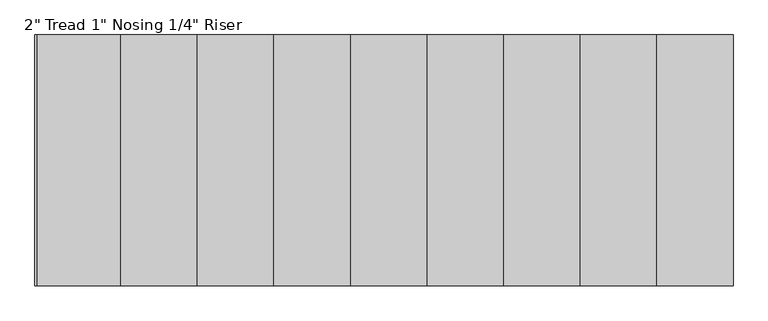
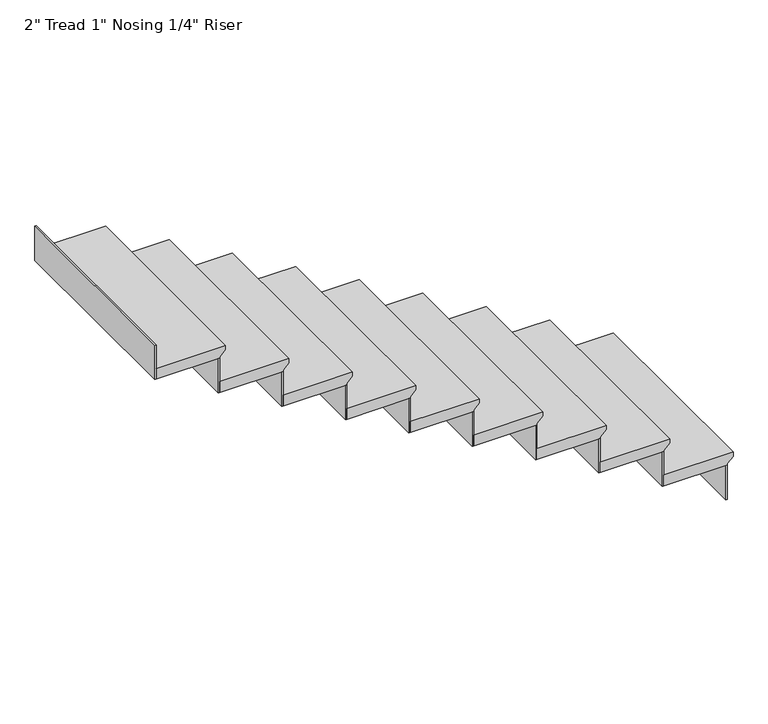
"""IFC4 building model written with IfcOpenShell, lengths in millimetres: stair flight geometry."""

from ifc_helpers import new_model, si_unit, frame, origin, place, context, project, spatial, polyline, outline, extrude, source, transform, mapped, element, save


def stair_flight_035a5224(model_context):
    return source(origin(), model_context, "Body", "SweptSolid", [
        extrude(outline(polyline([(1760.22, 923.4845537), (1760.22, 618.6845537), (1709.42, 618.6845537), (1709.42, 898.0845537), (1715.77, 898.0845537), (1741.17, 923.4845537), (1760.22, 923.4845537)])), frame((0.0, -5753.3544725, 0.0), z_axis=(0.0, 1.0, 0.0), x_axis=(0.0, 0.0, 1.0)), (0.0, 0.0, 1.0), 914.4),
        extrude(outline(polyline([(891.7345537, -4838.9544725), (898.0845537, -4838.9544725), (898.0845537, -5753.3544725), (891.7345537, -5753.3544725), (891.7345537, -4838.9544725)])), frame((0.0, 0.0, 1549.4), z_axis=(0.0, 0.0, 1.0), x_axis=(1.0, 0.0, 0.0)), (0.0, 0.0, 1.0), 160.02),
        extrude(outline(polyline([(612.3345537, -4838.9544725), (618.6845537, -4838.9544725), (618.6845537, -5753.3544725), (612.3345537, -5753.3544725), (612.3345537, -4838.9544725)])), frame((0.0, 0.0, 1709.42), z_axis=(0.0, 0.0, 1.0), x_axis=(1.0, 0.0, 0.0)), (0.0, 0.0, 1.0), 160.02),
        extrude(outline(polyline([(1920.24, 644.0845537), (1920.24, 339.2845537), (1869.44, 339.2845537), (1869.44, 618.6845537), (1875.79, 618.6845537), (1901.19, 644.0845537), (1920.24, 644.0845537)])), frame((0.0, -5753.3544725, 0.0), z_axis=(0.0, 1.0, 0.0), x_axis=(0.0, 0.0, 1.0)), (0.0, 0.0, 1.0), 914.4),
        extrude(outline(polyline([(332.9345537, -4838.9544725), (339.2845537, -4838.9544725), (339.2845537, -5753.3544725), (332.9345537, -5753.3544725), (332.9345537, -4838.9544725)])), frame((0.0, 0.0, 1869.44), z_axis=(0.0, 0.0, 1.0), x_axis=(1.0, 0.0, 0.0)), (0.0, 0.0, 1.0), 160.02),
        extrude(outline(polyline([(2080.26, 364.6845537), (2080.26, 59.8845537), (2029.46, 59.8845537), (2029.46, 339.2845537), (2035.81, 339.2845537), (2061.21, 364.6845537), (2080.26, 364.6845537)])), frame((0.0, -5753.3544725, 0.0), z_axis=(0.0, 1.0, 0.0), x_axis=(0.0, 0.0, 1.0)), (0.0, 0.0, 1.0), 914.4),
        extrude(outline(polyline([(53.5345537, -4838.9544725), (59.8845537, -4838.9544725), (59.8845537, -5753.3544725), (53.5345537, -5753.3544725), (53.5345537, -4838.9544725)])), frame((0.0, 0.0, 2029.46), z_axis=(0.0, 0.0, 1.0), x_axis=(1.0, 0.0, 0.0)), (0.0, 0.0, 1.0), 160.02),
        extrude(outline(polyline([(2240.28, 85.2845537), (2240.28, -219.5154463), (2189.48, -219.5154463), (2189.48, 59.8845537), (2195.83, 59.8845537), (2221.23, 85.2845537), (2240.28, 85.2845537)])), frame((0.0, -5753.3544725, 0.0), z_axis=(0.0, 1.0, 0.0), x_axis=(0.0, 0.0, 1.0)), (0.0, 0.0, 1.0), 914.4),
        extrude(outline(polyline([(-225.8654463, -4838.9544725), (-219.5154463, -4838.9544725), (-219.5154463, -5753.3544725), (-225.8654463, -5753.3544725), (-225.8654463, -4838.9544725)])), frame((0.0, 0.0, 2189.48), z_axis=(0.0, 0.0, 1.0), x_axis=(1.0, 0.0, 0.0)), (0.0, 0.0, 1.0), 160.02),
        extrude(outline(polyline([(2400.3, -194.1154463), (2400.3, -498.9154463), (2349.5, -498.9154463), (2349.5, -219.5154463), (2355.85, -219.5154463), (2381.25, -194.1154463), (2400.3, -194.1154463)])), frame((0.0, -5753.3544725, 0.0), z_axis=(0.0, 1.0, 0.0), x_axis=(0.0, 0.0, 1.0)), (0.0, 0.0, 1.0), 914.4),
        extrude(outline(polyline([(-505.2654463, -4838.9544725), (-498.9154463, -4838.9544725), (-498.9154463, -5753.3544725), (-505.2654463, -5753.3544725), (-505.2654463, -4838.9544725)])), frame((0.0, 0.0, 2349.5), z_axis=(0.0, 0.0, 1.0), x_axis=(1.0, 0.0, 0.0)), (0.0, 0.0, 1.0), 160.02),
        extrude(outline(polyline([(2560.32, -473.5154463), (2560.32, -778.3154463), (2509.52, -778.3154463), (2509.52, -498.9154463), (2515.87, -498.9154463), (2541.27, -473.5154463), (2560.32, -473.5154463)])), frame((0.0, -5753.3544725, 0.0), z_axis=(0.0, 1.0, 0.0), x_axis=(0.0, 0.0, 1.0)), (0.0, 0.0, 1.0), 914.4),
        extrude(outline(polyline([(-784.6654463, -4838.9544725), (-778.3154463, -4838.9544725), (-778.3154463, -5753.3544725), (-784.6654463, -5753.3544725), (-784.6654463, -4838.9544725)])), frame((0.0, 0.0, 2509.52), z_axis=(0.0, 0.0, 1.0), x_axis=(1.0, 0.0, 0.0)), (0.0, 0.0, 1.0), 160.02),
        extrude(outline(polyline([(2720.34, -752.9154463), (2720.34, -1057.7154463), (2669.54, -1057.7154463), (2669.54, -778.3154463), (2675.89, -778.3154463), (2701.29, -752.9154463), (2720.34, -752.9154463)])), frame((0.0, -5753.3544725, 0.0), z_axis=(0.0, 1.0, 0.0), x_axis=(0.0, 0.0, 1.0)), (0.0, 0.0, 1.0), 914.4),
        extrude(outline(polyline([(-1064.0654463, -4838.9544725), (-1057.7154463, -4838.9544725), (-1057.7154463, -5753.3544725), (-1064.0654463, -5753.3544725), (-1064.0654463, -4838.9544725)])), frame((0.0, 0.0, 2669.54), z_axis=(0.0, 0.0, 1.0), x_axis=(1.0, 0.0, 0.0)), (0.0, 0.0, 1.0), 160.02),
        extrude(outline(polyline([(2880.36, -1032.3154463), (2880.36, -1337.1154463), (2829.56, -1337.1154463), (2829.56, -1057.7154463), (2835.91, -1057.7154463), (2861.31, -1032.3154463), (2880.36, -1032.3154463)])), frame((0.0, -5753.3544725, 0.0), z_axis=(0.0, 1.0, 0.0), x_axis=(0.0, 0.0, 1.0)), (0.0, 0.0, 1.0), 914.4),
        extrude(outline(polyline([(-1343.4654463, -4838.9544725), (-1337.1154463, -4838.9544725), (-1337.1154463, -5753.3544725), (-1343.4654463, -5753.3544725), (-1343.4654463, -4838.9544725)])), frame((0.0, 0.0, 2829.56), z_axis=(0.0, 0.0, 1.0), x_axis=(1.0, 0.0, 0.0)), (0.0, 0.0, 1.0), 160.02),
        extrude(outline(polyline([(-1622.8654463, -4838.9544725), (-1616.5154463, -4838.9544725), (-1616.5154463, -5753.3544725), (-1622.8654463, -5753.3544725), (-1622.8654463, -4838.9544725)])), frame((0.0, 0.0, 2989.58), z_axis=(0.0, 0.0, 1.0), x_axis=(1.0, 0.0, 0.0)), (0.0, 0.0, 1.0), 160.02),
        extrude(outline(polyline([(3040.38, -1311.7154463), (3040.38, -1616.5154463), (2989.58, -1616.5154463), (2989.58, -1337.1154463), (2995.93, -1337.1154463), (3021.33, -1311.7154463), (3040.38, -1311.7154463)])), frame((0.0, -5753.3544725, 0.0), z_axis=(0.0, 1.0, 0.0), x_axis=(0.0, 0.0, 1.0)), (0.0, 0.0, 1.0), 914.4),
    ])


if __name__ == "__main__":
    model = new_model("IFC4")
    model_context = context("Model", 3, world=origin())
    ifc_project = project(units=[si_unit("LENGTHUNIT", "METRE", prefix="MILLI")], contexts=[model_context])
    site = spatial("IfcSite", under=ifc_project)
    building = spatial("IfcBuilding", under=site)
    placement = place(None, origin())
    stair_flight_shape = stair_flight_035a5224(model_context)
    element("IfcStairFlight", 1, ObjectType="2\" Tread 1\" Nosing 1/4\" Riser", at=placement, inside=building, context=model_context, shape_type="MappedRepresentation", body=[
        mapped(stair_flight_shape, transform((0.0, 0.0, 0.0), x_axis=(1.0, 0.0, 0.0), y_axis=(0.0, 1.0, 0.0), z_axis=(0.0, 0.0, 1.0))),
    ])
    save(model, "model.ifc")
